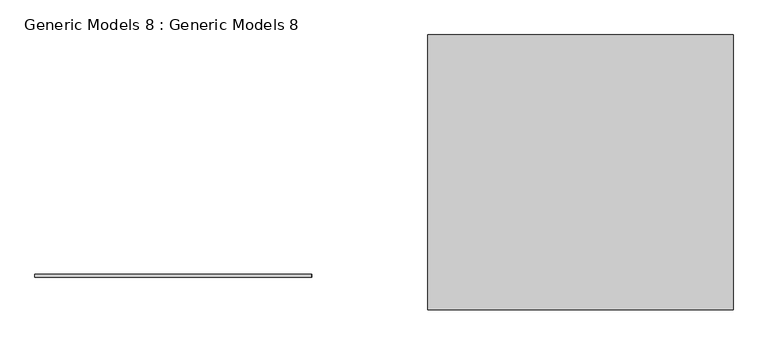
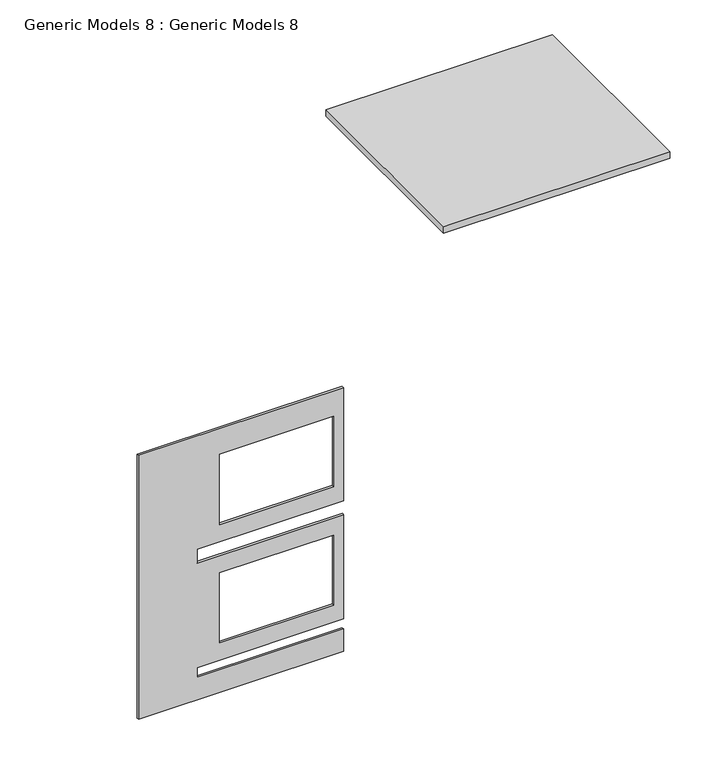
"""IFC4 building model written with IfcOpenShell, lengths in millimetres: proxy geometry, Generic Models 8 : Generic Models 8."""

from ifc_helpers import new_model, si_unit, frame, origin, place, context, project, spatial, polyline, outline, extrude, faceted_brep, source, transform, mapped, element, save


def generic_models_8_generic_models_8_0a5f4393(model_context):
    return source(origin(), model_context, "Body", "SolidModel", [
        faceted_brep([(-12889.5926394, -14185.5752569, 9144.0), (-17543.4695233, -14185.5752569, 9144.0), (-17543.4695233, -14185.5752569, 2812.195855), (-12886.9719936, -14185.5752569, 2812.195855), (-12886.9719936, -14185.5752569, 3352.8), (-16217.2212454, -14185.5752569, 3352.8), (-16217.2212454, -14185.5752569, 3588.5355704), (-12884.8411453, -14185.5752569, 3588.5355704), (-12884.8411453, -14185.5752569, 6096.0), (-16217.2212454, -14185.5752569, 6096.0), (-16217.2212454, -14185.5752569, 6429.1436541), (-12889.5531477, -14185.5752569, 6429.1436541), (-15701.9695233, -14185.5752569, 8530.8973501), (-13111.1695233, -14185.5752569, 8530.8973501), (-13111.1695233, -14185.5752569, 6841.9204311), (-15701.9695233, -14185.5752569, 6841.9204311), (-15701.9695233, -14185.5752569, 5678.6814593), (-13111.1695233, -14185.5752569, 5678.6814593), (-13111.1695233, -14185.5752569, 4001.8016497), (-15701.9695233, -14185.5752569, 4001.8016497), (-17543.4695233, -14134.7752569, 9144.0), (-12889.5926394, -14134.7752569, 9144.0), (-12889.5531477, -14134.7752569, 6429.1436541), (-16217.2212454, -14134.7752569, 6429.1436541), (-16217.2212454, -14134.7752569, 6096.0), (-12884.8411453, -14134.7752569, 6096.0), (-12884.8411453, -14134.7752569, 3588.5355704), (-16217.2212454, -14134.7752569, 3588.5355704), (-16217.2212454, -14134.7752569, 3352.8), (-12886.9719936, -14134.7752569, 3352.8), (-12886.9719936, -14134.7752569, 2812.195855), (-17543.4695233, -14134.7752569, 2812.195855), (-13111.1695233, -14134.7752569, 8530.8973501), (-15701.9695233, -14134.7752569, 8530.8973501), (-15701.9695233, -14134.7752569, 6841.9204311), (-13111.1695233, -14134.7752569, 6841.9204311), (-13111.1695233, -14134.7752569, 5678.6814593), (-15701.9695233, -14134.7752569, 5678.6814593), (-15701.9695233, -14134.7752569, 4001.8016497), (-13111.1695233, -14134.7752569, 4001.8016497)], [[[0, 1, 2, 3, 4, 5, 6, 7, 8, 9, 10, 11], [12, 13, 14, 15], [16, 17, 18, 19]], [[20, 21, 22, 23, 24, 25, 26, 27, 28, 29, 30, 31], [32, 33, 34, 35], [36, 37, 38, 39]], [[20, 1, 0, 21]], [[1, 20, 31, 2]], [[22, 11, 10, 23]], [[33, 12, 15, 34]], [[12, 33, 32, 13]], [[21, 0, 11, 22]], [[13, 32, 35, 14]], [[3, 2, 31, 30]], [[23, 10, 9, 24]], [[27, 6, 5, 28]], [[9, 8, 25, 24]], [[16, 37, 36, 17]], [[25, 8, 7, 26]], [[6, 27, 26, 7]], [[37, 16, 19, 38]], [[15, 14, 35, 34]], [[17, 36, 39, 18]], [[19, 18, 39, 38]], [[5, 4, 29, 28]], [[4, 3, 30, 29]]]),
        extrude(outline(polyline([(-10926.7695233, -10107.9295885), (-5790.2301761, -10107.9295885), (-5790.2301761, -14731.6752569), (-10926.7695233, -14731.6752569), (-10926.7695233, -10107.9295885)])), frame((0.0, 0.0, 12496.8), z_axis=(0.0, 0.0, 1.0), x_axis=(1.0, 0.0, 0.0)), (0.0, 0.0, 1.0), 152.4),
    ])


if __name__ == "__main__":
    model = new_model("IFC4")
    model_context = context("Model", 3, world=origin())
    ifc_project = project(units=[si_unit("LENGTHUNIT", "METRE", prefix="MILLI")], contexts=[model_context])
    site = spatial("IfcSite", under=ifc_project)
    building = spatial("IfcBuilding", under=site)
    placement = place(None, origin())
    generic_models_8_generic_models_8_shape = generic_models_8_generic_models_8_0a5f4393(model_context)
    element("IfcBuildingElementProxy", 1, Name="Generic Models 8 : Generic Models 8", ObjectType="Generic Models 8 : Generic Models 8", at=placement, inside=building, context=model_context, shape_type="MappedRepresentation", body=[
        mapped(generic_models_8_generic_models_8_shape, transform((0.0, 0.0, 0.0), x_axis=(1.0, 0.0, 0.0), y_axis=(0.0, 1.0, 0.0), z_axis=(0.0, 0.0, 1.0))),
    ])
    save(model, "model.ifc")
